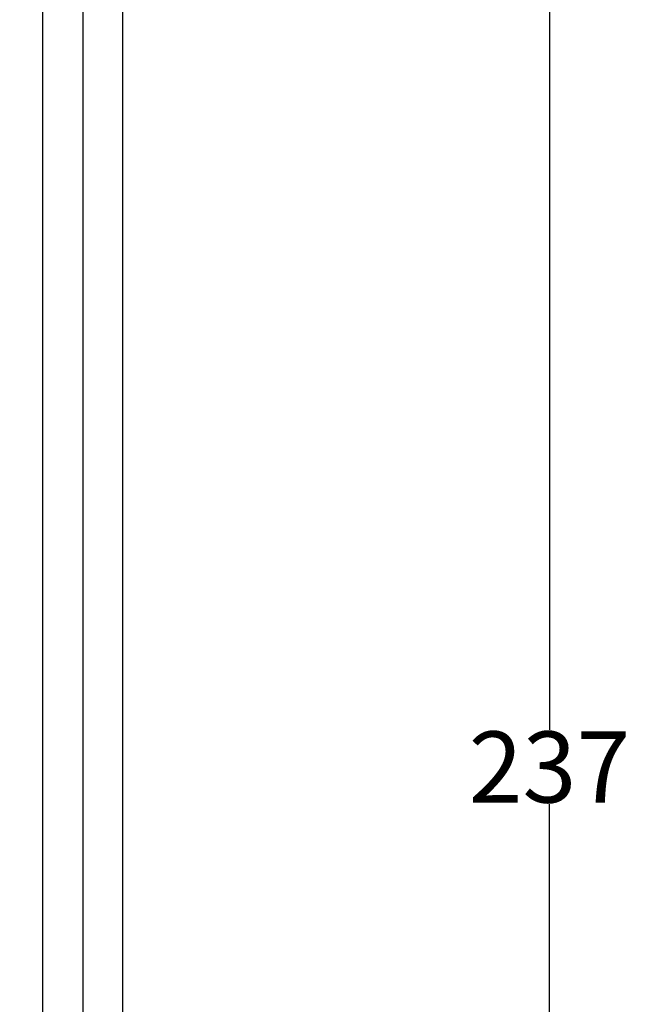
# Model space of a CAD drawing. Units: inches. Extents: x -48 to 50072, y 0 to 21068.
# Tile 44 of 75: x 542 to 611, y 306 to 417. Entities that reach past the tile are written whole.
import ezdxf

# ---------------------------------------------------------------- set-up
doc = ezdxf.new("R2010")
doc.units = ezdxf.units.IN
doc.header["$MEASUREMENT"] = 0
doc.linetypes.add('ACAD_ISO02W100', pattern=[15, 12, -3])
for name, color, linetype, lineweight in [('A-ANNO-DIMS', 2, 'Continuous', 18), ('C-PROP', 7, 'Continuous', 25), ('C-PROP-REF', 32, 'ACAD_ISO02W100', 13)]:
    doc.layers.add(name, color=color, linetype=linetype, lineweight=lineweight)
doc.styles.get("Standard").update_dxf_attribs({"font": 'arial.ttf'})
doc.dimstyles.get("Standard").update_dxf_attribs({"dimtxt": 8, "dimasz": 0.18, "dimexe": 0.18, "dimexo": 0.0625, "dimgap": 0.09, "dimtad": 0, "dimtih": 1, "dimtoh": 1, "dimdec": 1, "dimzin": 0, "dimdsep": 46, "dimlunit": 4, "dimtxsty": 'Standard', "dimblk": 'ARCHTICK', "dimcen": 0.09, "dimadec": 0, "dimazin": 0, "dimtfac": 1, "dimtdec": 1, "dimtofl": 0, "dimtmove": 0, "dimatfit": 3, "dimldrblk": 'ARCHTICK', "dimfxl": 1, "dimtolj": 1, "dimtzin": 0, "dimarcsym": 0})

# ---------------------------------------------------------------- blocks, each defined once
blk = doc.blocks.new('_ArchTick')
at = {"color": 0, "linetype": 'ByBlock', "const_width": 0.15}
blk.add_lwpolyline([(-0.5, -0.5), (0.5, 0.5)], dxfattribs=at)
blk = doc.blocks.new('*D115')
at = {"layer": 'A-ANNO-DIMS', "color": 0, "lineweight": -2, "transparency": 16777216}
for p, q in [((549.08, 451.07), (601.65, 451.07)), ((601.47, 451.07), (601.47, 336.75)), ((601.47, 214.07), (601.47, 328.4)), ((553.58, 214.07), (601.65, 214.07))]:
    blk.add_line(p, q, dxfattribs=at)
at = {"layer": 'Defpoints', "color": 0, "transparency": 16777216}
for p in [(549.02, 451.07), (601.47, 451.07), (553.52, 214.07)]:
    blk.add_point(p, dxfattribs=at)
at = {"layer": 'A-ANNO-DIMS', "color": 0, "lineweight": -2, "transparency": 16777216, "xscale": 0.18, "yscale": 0.18, "zscale": 0.18}
for p, rotation in [((601.47, 451.07), 90), ((601.47, 214.07), 270)]:
    blk.add_blockref('_ArchTick', p, dxfattribs=dict(at, rotation=rotation))
at = {"layer": 'A-ANNO-DIMS', "color": 0, "transparency": 16777216, "insert": (601.47, 332.57), "char_height": 8, "attachment_point": 5}
blk.add_mtext('\\A1;237', dxfattribs=at)
blk = doc.blocks.new('*D119')
at = {"layer": 'A-ANNO-DIMS', "color": 0, "lineweight": -2, "transparency": 16777216}
for p, q in [((463.52, 451.01), (463.52, 165.94)), ((549.02, 451.01), (549.02, 165.94)), ((463.52, 166.12), (495.75, 166.12)), ((549.02, 166.12), (516.78, 166.12))]:
    blk.add_line(p, q, dxfattribs=at)
at = {"layer": 'Defpoints', "color": 0, "transparency": 16777216}
for p in [(463.52, 451.07), (549.02, 451.07), (549.02, 166.12)]:
    blk.add_point(p, dxfattribs=at)
at = {"layer": 'A-ANNO-DIMS', "color": 0, "lineweight": -2, "transparency": 16777216, "xscale": 0.18, "yscale": 0.18, "zscale": 0.18, "rotation": 180}
blk.add_blockref('_ArchTick', (463.52, 166.12), dxfattribs=at)
at = {"layer": 'A-ANNO-DIMS', "color": 0, "lineweight": -2, "transparency": 16777216, "xscale": 0.18, "yscale": 0.18, "zscale": 0.18}
blk.add_blockref('_ArchTick', (549.02, 166.12), dxfattribs=at)
at = {"layer": 'A-ANNO-DIMS', "color": 0, "transparency": 16777216, "insert": (506.27, 166.12), "char_height": 8, "attachment_point": 5}
blk.add_mtext('\\A1;85.5', dxfattribs=at)

msp = doc.modelspace()

# ---------------------------------------------------------------- linework, layer by layer
at = {"layer": 'C-PROP'}
for p, q in [((553.517, 214.075), (553.517, 1170.775)), ((544.517, 223.075), (544.517, 488.775))]:
    msp.add_line(p, q, dxfattribs=at)
at = {"layer": 'C-PROP-REF'}
msp.add_line((549.017, 214.075), (549.017, 1166.275), dxfattribs=at)

# ---------------------------------------------------------------- dimensions: what is measured, and where the dimension line sits
at = {"layer": 'A-ANNO-DIMS'}
dim = msp.add_linear_dim(base=(549.017, 166.125), p1=(463.517, 451.075), p2=(549.017, 451.075), dimstyle='Standard', override={"dimdec": 1, "dimlfac": 1, "dimrnd": 0, "dimzin": 0, "dimdsep": 46, "dimlunit": 2}, dxfattribs=at)
dim.commit()
dim.dimension.update_dxf_attribs({"geometry": '*D119', "text_midpoint": (506.267, 166.125)})
dim = msp.add_linear_dim(base=(601.467, 451.075), p1=(553.517, 214.075), p2=(549.017, 451.075), angle=90, dimstyle='Standard', override={"dimdec": 0, "dimlfac": 1, "dimrnd": 0, "dimzin": 0, "dimdsep": 46, "dimlunit": 2}, dxfattribs=at)
dim.commit()
dim.dimension.update_dxf_attribs({"geometry": '*D115', "text_midpoint": (601.467, 332.575)})

doc.saveas('drawing.dxf')
